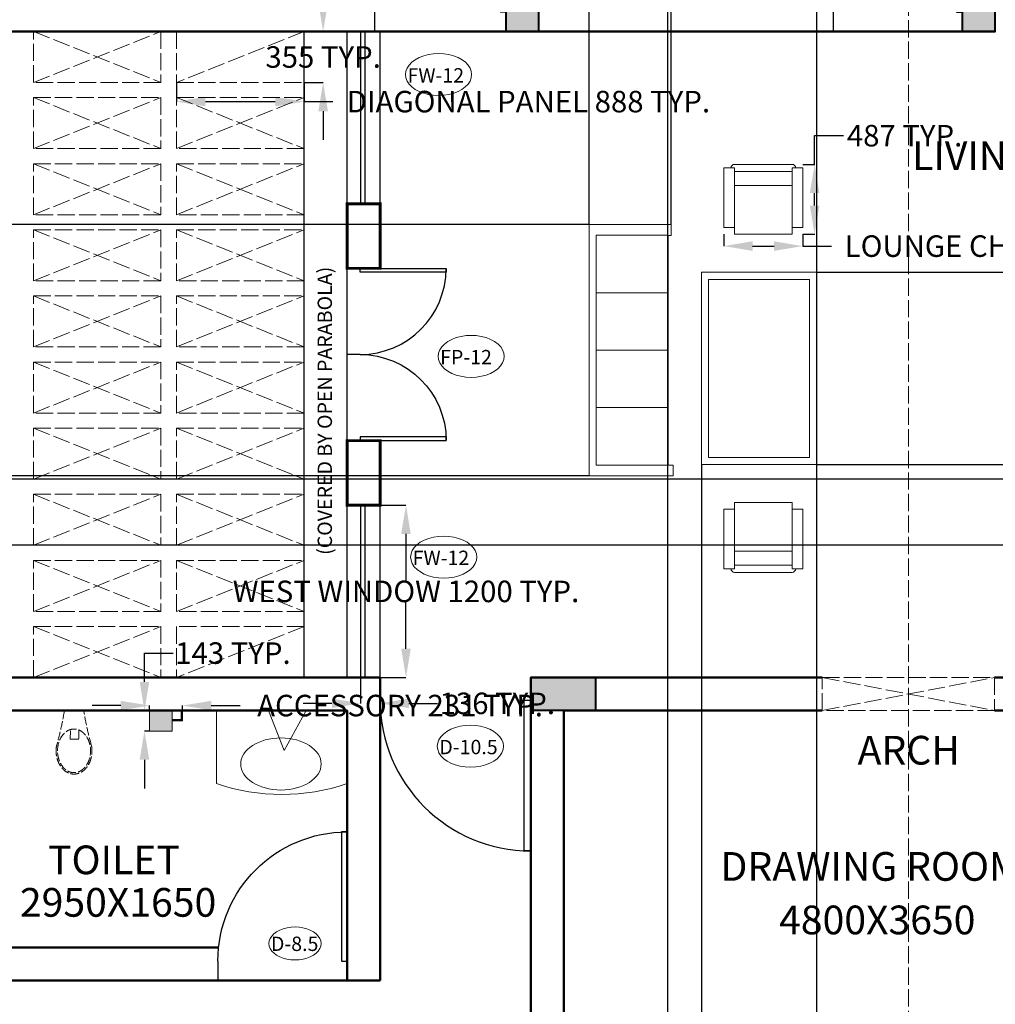
# Model space of a CAD drawing. Units: inches. Extents: x 22626 to 57351, y 2118 to 36234.
# Tile 4 of 10: x 34432 to 41227, y 16521 to 23379. Entities that reach past the tile are written whole.
import ezdxf

# ---------------------------------------------------------------- set-up
doc = ezdxf.new("R2010")
doc.units = ezdxf.units.IN
doc.header["$MEASUREMENT"] = 0
doc.linetypes.add('ACAD_ISO02W100', pattern=[15, 12, -3])
for name, color, linetype, lineweight in [('A-ANNO-DIMS', 130, 'Continuous', 18), ('A-ANNO-IDEN', 130, 'Continuous', 15), ('A-ANNO-TEXT', 130, 'Continuous', 18), ('A-AREA-IDEN', 130, 'Continuous', 18), ('A-COLS', 7, 'Continuous', 40), ('A-DOOR-OVHD', 32, 'ACAD_ISO02W100', 18), ('A-FLOR-FIXT', 30, 'Continuous', 18), ('A-FLOR-FIXT-HIDN', 30, 'ACAD_ISO02W100', 18), ('A-ROOF', 80, 'Continuous', 25), ('A-ROOF-OVHD', 80, 'ACAD_ISO02W100', 18), ('A-WALL', 80, 'Continuous', 50), ('DOORS', 32, 'Continuous', 25), ('FURNITURE', 30, 'Continuous', 18), ('WINDOWS', 212, 'Continuous', 25)]:
    doc.layers.add(name, color=color, linetype=linetype, lineweight=lineweight)
doc.layers.add('A-SECT', color=2, linetype='ACAD_ISO02W100', lineweight=18, true_color=0xf1eb1f)
doc.styles.get("Standard").update_dxf_attribs({"font": 'arial.ttf'})
doc.dimstyles.get("Standard").update_dxf_attribs({"dimtxt": 150, "dimasz": 200, "dimexe": 0.18, "dimexo": 0.0625, "dimgap": 0.09, "dimtad": 0, "dimtih": 1, "dimtoh": 1, "dimdec": 0, "dimzin": 0, "dimdsep": 46, "dimtxsty": 'Standard', "dimcen": 0.09, "dimadec": 0, "dimazin": 0, "dimtfac": 1, "dimtdec": 0, "dimtofl": 0, "dimtmove": 0, "dimatfit": 3, "dimfxl": 1, "dimtolj": 1, "dimtzin": 0, "dimarcsym": 0})

# ---------------------------------------------------------------- blocks, each defined once
blk = doc.blocks.new('*U7')
for p, q in [((0, 0), (-1e-16, -5.999999999999999)), ((40, -6e-16), (40, -6))]:
    blk.add_line(p, q)
blk.add_lwpolyline([(0, 0), (5.6e-15, 40), (1.750000000000007, 40), (1.749999999999998, -7e-16)], close=True)
blk.add_arc((0, 0), 40, 0, 90)
blk = doc.blocks.new('CHAIR-LOUNGE')
for p, q in [((475.0003983844144, 486.7758832616018), (75.00039838441444, 486.7758832616018)), ((0.0003983844144386, 47.37697057033074), (0.0003983844144386, 461.7758832616018)), ((75.00039838441444, 461.7758832616018), (0.0003983844144386, 461.7758832616018)), ((75.00039838441444, 461.7758832616018), (75.00039838441444, -4.78506444779e-05)), ((475.0003983844144, 436.7758832616018), (75.00039838441444, 436.7758832616018)), ((475.0003983844362, 461.7501739628424), (550.0003983844362, 461.7501739628424)), ((475.0003983844144, -4.78506444779e-05), (475.0003983844144, 461.750173962846)), ((550.0003983844144, 47.37697057033074), (550.0003983844144, 461.7501739628424)), ((75.00039838441444, 339.7687890747984), (475.0003983844144, 339.7687890747984)), ((75.00039838441444, 47.37697057033074), (0.0003983844144386, 47.37697057033074)), ((475.0003983844144, 47.37697057033074), (550.0003983844144, 47.37697057033074)), ((75.00039838440716, -4.78506481159e-05), (475.0003983844144, -4.78506481159e-05))]:
    blk.add_line(p, q)
for centre, start, end in [((75.00039838441444, 461.7758832616018), 90, 180), ((475.0003983844144, 461.7758832616018), 359.9410786171467, 90)]:
    blk.add_arc(centre, 25, start, end)
blk = doc.blocks.new('WC')
at = {"ltscale": 5}
for p, q in [((307.4540408789253, 157.9229967620813), (242.2174300020561, 157.9229967620813)), ((242.2174300020561, 157.9229967620813), (242.2174300020561, 97.87988847275483)), ((307.4540408789253, 157.9229967620813), (307.4540408789253, 157.9229967620813)), ((242.2174300020561, 97.87988847275483), (310.0842174796853, 99.70460823710528))]:
    blk.add_line(p, q, dxfattribs=at)
for centre, start, end in [((780.732508801062, 2286.288249576111), 254.000576969056, 260.8285458946419), ((780.732508801062, -2036.267674000785), 99.17145410535805, 105.999423030944)]:
    blk.add_arc(centre, 2121.236142909723, start, end, dxfattribs=at)
blk.add_ellipse((161.9027973060947, 125.0102877876634), major_axis=(151.9040759523413, 0), ratio=0.7571275708385353, start_param=-1.570796326794896, end_param=4.712388980384689, dxfattribs=at)
for points, knots in [([(196.0611207178517, 247.2193096078299), (189.9898489161132, 248.2266596507652), (183.8456655129121, 248.9650412442752), (168.6182293347155, 250.1102459839712), (159.4964975931143, 250.2034131541222), (141.3581357193834, 249.212698022955), (132.3417047420516, 248.1288311957833), (114.6613914742556, 244.8098406800164), (105.9976853845146, 242.5747636017513), (89.26201623554518, 237.0062334978611), (81.19018288652298, 233.6728365616509), (65.86452451616788, 225.9859897466813), (58.61077128878969, 221.6325587335632), (45.13156838521536, 212.0080719868456), (38.90616664764093, 206.7369257869286), (27.67640637096338, 195.4043234284545), (22.67220516936504, 189.3426231032536), (14.05759261523781, 176.5860631599644), (10.44766267286468, 169.8909471035294), (4.765577569938614, 156.0629077761186), (2.69424158098991, 148.9301527436837), (0.1846293913040426, 134.463597005164), (-0.2530317139462568, 127.1307025187488), (0.5271766823570943, 112.5265070110981), (1.744832412616233, 105.2563518462193), (5.77749157987273, 91.03263116568269), (8.591685077881264, 84.07962673572185), (15.69573821845551, 70.70922901844096), (19.98490811580268, 64.29173781119243), (29.87879523489392, 52.16900764399179), (35.483208879421, 46.46348057011346), (47.82439502190391, 35.90657261581146), (54.56108629030495, 31.05501885116246), (68.96556532807881, 22.32099587028279), (76.63330319123634, 18.43849746629348), (92.68186228567357, 11.73355477496807), (101.0625846676266, 8.91115468616772), (118.3043576900527, 4.392898517646244), (127.1652540279829, 2.697098106120392), (144.6597339432555, 0.5298149587142689), (153.2812269904534, -0.000476238605188), (161.9027973060947, -0.000476238605188)], [1.35503494441986, 1.35503494441986, 1.35503494441986, 1.35503494441986, 1.471789532681877, 1.471789532681877, 1.642812487519809, 1.642812487519809, 1.813835442357741, 1.813835442357741, 1.984858397195673, 1.984858397195673, 2.155881352033606, 2.155881352033606, 2.326904306871538, 2.326904306871538, 2.49792726170947, 2.49792726170947, 2.668950216547402, 2.668950216547402, 2.839973171385334, 2.839973171385334, 3.010996126223266, 3.010996126223266, 3.182019081061198, 3.182019081061198, 3.35304203589913, 3.35304203589913, 3.524064990737062, 3.524064990737062, 3.695087945574994, 3.695087945574994, 3.866110900412926, 3.866110900412926, 4.037133855250859, 4.037133855250859, 4.208156810088791, 4.208156810088791, 4.379179764926723, 4.379179764926723, 4.550202719764655, 4.550202719764655, 4.712388980384689, 4.712388980384689, 4.712388980384689, 4.712388980384689]), ([(161.9027973060947, -0.000476238605188), (167.8851873344465, -0.000476238605188), (173.8675648995122, 0.254611844480678), (185.2699231324077, 1.230286525809788), (190.6953945214336, 1.911114408936555), (196.0639028232108, 2.802063691000512)], [-1.570796326794896, -1.570796326794896, -1.570796326794896, -1.570796326794896, -1.458257493061962, -1.458257493061962, -1.355016516099114, -1.355016516099114, -1.355016516099114, -1.355016516099114])]:
    blk.add_open_spline(points, degree=3, knots=knots, dxfattribs=at)
blk = doc.blocks.new('VANITY-BASIN')
for p, q in [((584.7220439586453, 910.0402479339828), (75.43762569876708, 910.0402479339828)), ((305.8230790732414, 471.9850997598696), (584.7220439586453, 624.7406586797733)), ((305.8230790732414, 471.9850997598696), (584.7220439586453, 362.8739423048537))]:
    blk.add_line(p, q)
blk.add_arc((1409.991080111897, 455.0201781493488), 1409.991555504085, 161.1730336158717, 198.8269663841282)
blk.add_ellipse((212.5566461408889, 449.1359101998277), major_axis=(0, -280.3059750137254), ratio=0.6469075979310198)
blk = doc.blocks.new('COL-RECTANGULAR')
h = blk.add_hatch(color=256)
h.dxf.hatch_style = 1
h.paths.add_polyline_path([(4.39586474386e-05, 0.0001083647293854), (450.0000439586474, 0.0001083647293854), (450.0000439586474, 230.0001083647294), (4.39586474386e-05, 230.0001083647294)])
blk.add_lwpolyline([(4.39586474386e-05, 0.0001083647293854), (4.39586474386e-05, 230.0001083647294), (450.0000439586474, 230.0001083647294), (450.0000439586474, 0.0001083647293854)], close=True)
blk = doc.blocks.new('CANOPY-CROSSED-PANEL')
at = {"ltscale": 10}
for p, q in [((4.39586510765e-05, -7.7958175098e-06), (887.5000439586511, 355.3241083647299)), ((4.39586510765e-05, 355.3241083647299), (887.5000439586511, -7.7958175098e-06))]:
    blk.add_line(p, q, dxfattribs=at)
blk.add_lwpolyline([(4.39586510765e-05, 355.3241083647299), (887.5000439586511, 355.3241083647299), (887.5000439586511, -7.7958175098e-06), (4.39586510765e-05, -7.7958175098e-06)], close=True, dxfattribs=at)
blk = doc.blocks.new('BATH-WALL-ACCESSORY')
h = blk.add_hatch(color=256)
h.dxf.hatch_style = 1
h.paths.add_polyline_path([(142.8430439586445, 231.1050653827879), (71.42162994010141, 231.1050653827879), (71.42162994010141, 158.5160872540764), (81.4216299401014, 158.5160872540764), (81.42162994010869, 221.1050653827879), (142.8430439586445, 221.1050653827879)])
h = blk.add_hatch(color=256)
h.dxf.hatch_style = 1
h.paths.add_polyline_path([(142.8430439586445, 158.5160872540764), (0.0002159215582651, 158.5160872540764), (0.0002159215582651, -1.22242890939e-05), (142.8430439586445, -1.22242854559e-05)])
for p, q in [((71.42162994010141, 158.5160872540764), (71.42162994010141, 231.1050653827879)), ((71.42162994010141, 231.1050653827879), (142.8430439586445, 231.1050653827879)), ((81.42162994010869, 221.1050653827879), (142.8430439586445, 221.1050653827879)), ((81.4216299401014, 158.5160872540764), (81.42162994010869, 221.1050653827879)), ((142.8430439586445, 158.5160872540764), (0.0002159215582651, 158.5160872540764)), ((0.0002159215582651, 158.5160872540764), (0.0002159215582651, -1.22242890939e-05)), ((142.8430439586445, 158.5160872540764), (142.8430439586445, 158.5160872540764)), ((0.0002159215582651, -1.22242890939e-05), (142.8430439586445, -1.22242854559e-05))]:
    blk.add_line(p, q)
blk = doc.blocks.new('WIN-FIXED-1200-WEST')
for p, q in [((0.0004449870903045, 1200.000108364729), (0.0004449870903045, 0.0001083647293854)), ((30.0004449870903, 1200.000108364729), (30.0004449870903, 0.0001083647293854))]:
    blk.add_line(p, q)
blk.add_lwpolyline([(136.2710439586444, 0.0001083647293854), (136.2710439586444, 1200.000108364729)])
blk = doc.blocks.new('CANOPY-DIAGONAL-PANEL')
at = {"ltscale": 10}
blk.add_line((887.5000439586511, 355.3241083647299), (4.39586510765e-05, -7.7958175098e-06), dxfattribs=at)
blk.add_lwpolyline([(887.5000439586511, 355.3241083647299), (4.39586510765e-05, 355.3241083647299), (4.39586510765e-05, -7.7958175098e-06), (887.5000439586511, -7.7958175098e-06)], close=True, dxfattribs=at)
blk = doc.blocks.new('*D52')
at = {"layer": 'A-ANNO-DIMS', "color": 0, "lineweight": -2, "transparency": 16777216}
for p, q in [((35524.92904395865, 22941.47349220418), (35524.92904395865, 22808.23099220418)), ((36412.42904395865, 22941.47349220418), (36412.42904395865, 22808.23099220418)), ((35724.92904395865, 22808.41099220418), (36212.42904395865, 22808.41099220418)), ((36412.42904395865, 22808.41099220418), (36612.42904395865, 22808.41099220418))]:
    blk.add_line(p, q, dxfattribs=at)
at = {"layer": 'A-ANNO-DIMS', "color": 0, "transparency": 16777216}
for points in [[(35724.92904395865, 22841.74432553752), (35724.92904395865, 22775.07765887085), (35524.92904395865, 22808.41099220418)], [(36212.42904395865, 22841.74432553752), (36212.42904395865, 22775.07765887085), (36412.42904395865, 22808.41099220418)]]:
    blk.add_solid(points, dxfattribs=at)
at = {"layer": 'Defpoints', "color": 0, "transparency": 16777216}
for p in [(35524.92904395865, 22941.53599220418), (36412.42904395865, 22941.53599220418), (36412.42904395865, 22808.41099220418)]:
    blk.add_point(p, dxfattribs=at)
at = {"layer": 'A-ANNO-DIMS', "color": 0, "transparency": 16777216, "insert": (37975.41126769671, 22808.41099220418), "char_height": 150, "attachment_point": 5}
blk.add_mtext('\\A1;DIAGONAL PANEL 888 TYP.', dxfattribs=at)
blk = doc.blocks.new('*D53')
at = {"layer": 'A-ANNO-DIMS', "color": 0, "lineweight": -2, "transparency": 16777216}
for p, q in [((36545.55404395868, 23496.86010836474), (36545.55404395868, 23696.86010836474)), ((36412.49154395866, 23296.86010836474), (36545.73404395868, 23296.86010836474)), ((36412.49154395866, 22941.53599220419), (36545.73404395868, 22941.53599220419)), ((36545.55404395868, 22741.53599220419), (36545.55404395868, 22541.53599220419))]:
    blk.add_line(p, q, dxfattribs=at)
at = {"layer": 'A-ANNO-DIMS', "color": 0, "transparency": 16777216}
for points in [[(36512.22071062534, 23496.86010836474), (36578.88737729201, 23496.86010836474), (36545.55404395868, 23296.86010836474)], [(36512.22071062534, 22741.53599220419), (36578.88737729201, 22741.53599220419), (36545.55404395868, 22941.53599220419)]]:
    blk.add_solid(points, dxfattribs=at)
at = {"layer": 'Defpoints', "color": 0, "transparency": 16777216}
for p in [(36412.42904395866, 23296.86010836474), (36545.55404395868, 23296.86010836474), (36412.42904395866, 22941.53599220419)]:
    blk.add_point(p, dxfattribs=at)
at = {"layer": 'A-ANNO-DIMS', "color": 0, "transparency": 16777216, "insert": (36545.55404395868, 23119.19805028445), "char_height": 150, "attachment_point": 5}
blk.add_mtext('\\A1;355 TYP.', dxfattribs=at)
blk = doc.blocks.new('*D68')
at = {"layer": 'A-ANNO-DIMS', "color": 0, "lineweight": -2, "transparency": 16777216}
for p, q in [((35135.53720708872, 18601.52587000579), (34935.53720708872, 18601.52587000579)), ((35335.53720708872, 18566.92260836472), (35335.53720708872, 18601.70587000579)), ((35566.6422846958, 18566.92260836472), (35566.6422846958, 18601.70587000579)), ((35766.6422846958, 18601.52587000579), (35966.6422846958, 18601.52587000579))]:
    blk.add_line(p, q, dxfattribs=at)
at = {"layer": 'A-ANNO-DIMS', "color": 0, "transparency": 16777216}
for points in [[(35135.53720708872, 18634.85920333912), (35135.53720708872, 18568.19253667246), (35335.53720708872, 18601.52587000579)], [(35766.6422846958, 18634.85920333912), (35766.6422846958, 18568.19253667246), (35566.6422846958, 18601.52587000579)]]:
    blk.add_solid(points, dxfattribs=at)
at = {"layer": 'Defpoints', "color": 0, "transparency": 16777216}
for p in [(35566.6422846958, 18601.52587000579), (35335.53720708872, 18566.86010836472), (35566.6422846958, 18566.86010836472)]:
    blk.add_point(p, dxfattribs=at)
at = {"layer": 'A-ANNO-DIMS', "color": 0, "transparency": 16777216, "insert": (37081.44920147616, 18601.52587000579), "char_height": 150, "attachment_point": 5}
blk.add_mtext('\\A1;ACCESSORY 231 TYP.', dxfattribs=at)
blk = doc.blocks.new('*D69')
at = {"layer": 'A-ANNO-DIMS', "color": 0, "lineweight": -2, "transparency": 16777216}
for p, q in [((35300.87144544769, 18766.86010836473), (35300.87144544769, 18966.86010836473)), ((35300.87144544769, 18966.86010836473), (35500.87144544769, 18966.86010836473)), ((35335.47470708873, 18566.86010836473), (35300.69144544769, 18566.86010836473)), ((35335.47470708873, 18424.01728032765), (35300.69144544769, 18424.01728032765)), ((35300.87144544769, 18224.01728032765), (35300.87144544769, 18024.01728032765))]:
    blk.add_line(p, q, dxfattribs=at)
at = {"layer": 'A-ANNO-DIMS', "color": 0, "transparency": 16777216}
for points in [[(35267.53811211435, 18766.86010836473), (35334.20477878102, 18766.86010836473), (35300.87144544769, 18566.86010836473)], [(35267.53811211435, 18224.01728032765), (35334.20477878102, 18224.01728032765), (35300.87144544769, 18424.01728032765)]]:
    blk.add_solid(points, dxfattribs=at)
at = {"layer": 'Defpoints', "color": 0, "transparency": 16777216}
for p in [(35300.87144544769, 18566.86010836473), (35335.53720708873, 18566.86010836473), (35335.53720708873, 18424.01728032765)]:
    blk.add_point(p, dxfattribs=at)
at = {"layer": 'A-ANNO-DIMS', "color": 0, "transparency": 16777216, "insert": (35917.24725718029, 18966.86010836472), "char_height": 150, "attachment_point": 5}
blk.add_mtext('\\A1;143 TYP.', dxfattribs=at)
blk = doc.blocks.new('*D76')
at = {"layer": 'A-ANNO-DIMS', "color": 0, "lineweight": -2, "transparency": 16777216}
for p, q in [((39336.54639838442, 21884.32545214935), (39336.54639838442, 21801.70795214935)), ((39886.54639838444, 21884.32545214935), (39886.54639838444, 21801.70795214935)), ((39536.54639838442, 21801.88795214935), (39686.54639838444, 21801.88795214935)), ((39886.54639838444, 21801.88795214935), (40086.54639838444, 21801.88795214935))]:
    blk.add_line(p, q, dxfattribs=at)
at = {"layer": 'A-ANNO-DIMS', "color": 0, "transparency": 16777216}
for points in [[(39536.54639838442, 21835.22128548268), (39536.54639838442, 21768.55461881602), (39336.54639838442, 21801.88795214935)], [(39686.54639838444, 21835.22128548268), (39686.54639838444, 21768.55461881602), (39886.54639838444, 21801.88795214935)]]:
    blk.add_solid(points, dxfattribs=at)
at = {"layer": 'Defpoints', "color": 0, "transparency": 16777216}
for p in [(39336.54639838442, 21884.38795214935), (39886.54639838444, 21884.38795214935), (39886.54639838444, 21801.88795214935)]:
    blk.add_point(p, dxfattribs=at)
at = {"layer": 'A-ANNO-DIMS', "color": 0, "transparency": 16777216, "insert": (41333.34512962592, 21801.88795214935), "char_height": 150, "attachment_point": 5}
blk.add_mtext('\\A1;LOUNGE CHAIR 550 TYP.', dxfattribs=at)
blk = doc.blocks.new('*D77')
at = {"layer": 'A-ANNO-DIMS', "color": 0, "lineweight": -2, "transparency": 16777216}
for p, q in [((39969.04639838447, 22371.16388326161), (39969.04639838447, 22571.16388326161)), ((39969.04639838447, 22571.16388326161), (40169.04639838447, 22571.16388326161)), ((39886.60889838445, 22371.16388326161), (39969.22639838447, 22371.16388326161)), ((39969.04639838447, 22084.38795214936), (39969.04639838447, 22171.16388326161)), ((39886.60889838445, 21884.38795214936), (39969.22639838447, 21884.38795214936))]:
    blk.add_line(p, q, dxfattribs=at)
at = {"layer": 'A-ANNO-DIMS', "color": 0, "transparency": 16777216}
for points in [[(39935.71306505113, 22171.16388326161), (40002.3797317178, 22171.16388326161), (39969.04639838447, 22371.16388326161)], [(39935.71306505113, 22084.38795214936), (40002.3797317178, 22084.38795214936), (39969.04639838447, 21884.38795214936)]]:
    blk.add_solid(points, dxfattribs=at)
at = {"layer": 'Defpoints', "color": 0, "transparency": 16777216}
for p in [(39886.54639838446, 22371.16388326161), (39969.04639838447, 22371.16388326161), (39886.54639838446, 21884.38795214936)]:
    blk.add_point(p, dxfattribs=at)
at = {"layer": 'A-ANNO-DIMS', "color": 0, "transparency": 16777216, "insert": (40595.50065486468, 22571.1638832616), "char_height": 150, "attachment_point": 5}
blk.add_mtext('\\A1;487 TYP.', dxfattribs=at)
blk = doc.blocks.new('*D92')
at = {"layer": 'A-ANNO-DIMS', "color": 0, "lineweight": -2, "transparency": 16777216}
for p, q in [((36942.49154395866, 19996.86010836473), (37122.60904395868, 19996.86010836473)), ((37122.42904395868, 19796.86010836473), (37122.42904395868, 19474.55924888315)), ((37122.42904395868, 18996.86010836474), (37122.42904395868, 19319.16096784632)), ((36942.49154395866, 18796.86010836474), (37122.60904395868, 18796.86010836474))]:
    blk.add_line(p, q, dxfattribs=at)
at = {"layer": 'A-ANNO-DIMS', "color": 0, "transparency": 16777216}
for points in [[(37089.09571062534, 19796.86010836473), (37155.76237729201, 19796.86010836473), (37122.42904395868, 19996.86010836473)], [(37089.09571062534, 18996.86010836474), (37155.76237729201, 18996.86010836474), (37122.42904395868, 18796.86010836474)]]:
    blk.add_solid(points, dxfattribs=at)
at = {"layer": 'Defpoints', "color": 0, "transparency": 16777216}
for p in [(36942.42904395866, 19996.86010836473), (37122.42904395868, 19996.86010836473), (36942.42904395866, 18796.86010836474)]:
    blk.add_point(p, dxfattribs=at)
at = {"layer": 'A-ANNO-DIMS', "color": 0, "transparency": 16777216, "insert": (37122.42904395868, 19396.86010836472), "char_height": 150, "attachment_point": 5}
blk.add_mtext('\\A1;WEST WINDOW 1200 TYP.', dxfattribs=at)
blk = doc.blocks.new('*D93')
at = {"layer": 'A-ANNO-DIMS', "color": 0, "lineweight": -2, "transparency": 16777216}
for p, q in [((36806.1584449871, 18796.79760836473), (36806.1584449871, 18616.68010836473)), ((36942.42904395865, 18796.79760836473), (36942.42904395865, 18616.68010836473)), ((36606.1584449871, 18616.86010836473), (36406.1584449871, 18616.86010836473)), ((37142.42904395865, 18616.86010836473), (37342.42904395865, 18616.86010836473))]:
    blk.add_line(p, q, dxfattribs=at)
at = {"layer": 'A-ANNO-DIMS', "color": 0, "transparency": 16777216}
for points in [[(36606.1584449871, 18650.19344169806), (36606.1584449871, 18583.52677503139), (36806.1584449871, 18616.86010836473)], [(37142.42904395865, 18650.19344169806), (37142.42904395865, 18583.52677503139), (36942.42904395865, 18616.86010836473)]]:
    blk.add_solid(points, dxfattribs=at)
at = {"layer": 'Defpoints', "color": 0, "transparency": 16777216}
for p in [(36806.1584449871, 18796.86010836473), (36942.42904395865, 18796.86010836473), (36942.42904395865, 18616.86010836473)]:
    blk.add_point(p, dxfattribs=at)
at = {"layer": 'A-ANNO-DIMS', "color": 0, "transparency": 16777216, "insert": (37758.80485569126, 18616.86010836473), "char_height": 150, "attachment_point": 5}
blk.add_mtext('\\A1;136 TYP.', dxfattribs=at)
blk = doc.blocks.new('*D99')
at = {"layer": 'A-ANNO-DIMS', "color": 0, "lineweight": -2, "transparency": 16777216}
for p, q in [((41184.594559, 30456.86010800002), (57038.79342100006, 30456.86010800002)), ((57038.61342100005, 30256.86010800002), (57038.61342100005, 18933.58721577627)), ((57038.61342100006, 7456.860108000005), (57038.61342100005, 18780.13300022374)), ((43702.49154400001, 7256.860108000004), (57038.79342100006, 7256.860108000005))]:
    blk.add_line(p, q, dxfattribs=at)
at = {"layer": 'A-ANNO-DIMS', "color": 0, "transparency": 16777216}
for points in [[(57005.28008766672, 30256.86010800002), (57071.94675433339, 30256.86010800002), (57038.61342100005, 30456.86010800002)], [(57005.28008766673, 7456.860108000005), (57071.9467543334, 7456.860108000005), (57038.61342100006, 7256.860108000005)]]:
    blk.add_solid(points, dxfattribs=at)
at = {"layer": 'Defpoints', "color": 0, "transparency": 16777216}
for p in [(41184.53205900001, 30456.86010800002), (57038.61342100005, 30456.86010800002), (43702.42904400001, 7256.860108000004)]:
    blk.add_point(p, dxfattribs=at)
at = {"layer": 'A-ANNO-DIMS', "color": 0, "transparency": 16777216, "insert": (57038.61342100005, 18856.86010799999), "char_height": 150, "attachment_point": 5}
blk.add_mtext('\\A1;23200', dxfattribs=at)
blk = doc.blocks.new('*D100')
at = {"layer": 'A-ANNO-DIMS', "color": 0, "lineweight": -2, "transparency": 16777216}
for p, q in [((32057.429044, 23296.797608), (32057.429044, 2216.185148)), ((49187.429044, 23296.797608), (49187.429044, 2216.185148)), ((32257.429044, 2216.365148), (40347.407256824, 2216.365148)), ((48987.42904399999, 2216.365148), (40897.45083117598, 2216.365148))]:
    blk.add_line(p, q, dxfattribs=at)
at = {"layer": 'A-ANNO-DIMS', "color": 0, "transparency": 16777216}
for points in [[(32257.429044, 2249.698481333334), (32257.429044, 2183.031814666666), (32057.429044, 2216.365148)], [(48987.42904399999, 2249.698481333334), (48987.42904399999, 2183.031814666666), (49187.429044, 2216.365148)]]:
    blk.add_solid(points, dxfattribs=at)
at = {"layer": 'Defpoints', "color": 0, "transparency": 16777216}
for p in [(32057.429044, 23296.860108), (49187.429044, 23296.860108), (49187.429044, 2216.365148)]:
    blk.add_point(p, dxfattribs=at)
at = {"layer": 'A-ANNO-DIMS', "color": 0, "transparency": 16777216, "insert": (40622.42904399999, 2216.365148), "char_height": 150, "attachment_point": 5}
blk.add_mtext('\\A1;17130', dxfattribs=at)
blk = doc.blocks.new('*D104')
at = {"layer": 'A-ANNO-DIMS', "color": 0, "lineweight": -2, "transparency": 16777216}
for p, q in [((39180.506596, 20280.329385), (39180.506596, 2216.185148)), ((39982.977522, 20280.329385), (39982.977522, 2216.185148)), ((38980.506596, 2216.365148), (38780.506596, 2216.365148)), ((40182.977522, 2216.365148), (40382.977522, 2216.365148))]:
    blk.add_line(p, q, dxfattribs=at)
at = {"layer": 'A-ANNO-DIMS', "color": 0, "transparency": 16777216}
for points in [[(38980.506596, 2249.698481333334), (38980.506596, 2183.031814666666), (39180.506596, 2216.365148)], [(40182.977522, 2249.698481333334), (40182.977522, 2183.031814666666), (39982.977522, 2216.365148)]]:
    blk.add_solid(points, dxfattribs=at)
at = {"layer": 'Defpoints', "color": 0, "transparency": 16777216}
for p in [(39180.506596, 20280.391885), (39982.977522, 20280.391885), (39982.977522, 2216.365148)]:
    blk.add_point(p, dxfattribs=at)
at = {"layer": 'A-ANNO-DIMS', "color": 0, "transparency": 16777216, "insert": (39581.742059, 2216.365148), "char_height": 150, "attachment_point": 5}
blk.add_mtext('\\A1;802.5', dxfattribs=at)
blk = doc.blocks.new('*D105')
at = {"layer": 'A-ANNO-DIMS', "color": 0, "lineweight": -2, "transparency": 16777216}
for p, q in [((39983.04002200002, 21620.08858600001), (57038.79342100006, 21620.08858600001)), ((57038.61342100005, 21420.08858600001), (57038.61342100005, 21026.96734327627)), ((57038.61342100005, 20480.39188500001), (57038.61342100005, 20873.51312772375)), ((39983.04002200002, 20280.39188500001), (57038.79342100006, 20280.39188500001))]:
    blk.add_line(p, q, dxfattribs=at)
at = {"layer": 'A-ANNO-DIMS', "color": 0, "transparency": 16777216}
for points in [[(57005.28008766672, 21420.08858600001), (57071.94675433339, 21420.08858600001), (57038.61342100005, 21620.08858600001)], [(57005.28008766672, 20480.39188500001), (57071.94675433339, 20480.39188500001), (57038.61342100005, 20280.39188500001)]]:
    blk.add_solid(points, dxfattribs=at)
at = {"layer": 'Defpoints', "color": 0, "transparency": 16777216}
for p in [(39982.97752200002, 21620.08858600001), (57038.61342100005, 21620.08858600001), (39982.97752200002, 20280.39188500001)]:
    blk.add_point(p, dxfattribs=at)
at = {"layer": 'A-ANNO-DIMS', "color": 0, "transparency": 16777216, "insert": (57038.61342100005, 20950.24023549999), "char_height": 150, "attachment_point": 5}
blk.add_mtext('\\A1;1339.7', dxfattribs=at)
blk = doc.blocks.new('*D106')
at = {"layer": 'A-ANNO-DIMS', "color": 0, "lineweight": -2, "transparency": 16777216}
for p, q in [((38198.278783, 36136.059266), (37998.278783, 36136.059266)), ((38398.278783, 21952.121016), (38398.278783, 36136.239266)), ((38968.927296, 21952.121016), (38968.927296, 36136.239266)), ((39168.927296, 36136.059266), (39368.927296, 36136.059266))]:
    blk.add_line(p, q, dxfattribs=at)
at = {"layer": 'A-ANNO-DIMS', "color": 0, "transparency": 16777216}
for points in [[(38198.278783, 36169.39259933333), (38198.278783, 36102.72593266666), (38398.278783, 36136.059266)], [(39168.927296, 36169.39259933333), (39168.927296, 36102.72593266666), (38968.927296, 36136.059266)]]:
    blk.add_solid(points, dxfattribs=at)
at = {"layer": 'Defpoints', "color": 0, "transparency": 16777216}
for p in [(38968.927296, 36136.059266), (38398.278783, 21952.058516), (38968.927296, 21952.058516)]:
    blk.add_point(p, dxfattribs=at)
at = {"layer": 'A-ANNO-DIMS', "color": 0, "transparency": 16777216, "insert": (38683.6030395, 36136.059266), "char_height": 150, "attachment_point": 5}
blk.add_mtext('\\A1;570.6', dxfattribs=at)
blk = doc.blocks.new('*D107')
at = {"layer": 'A-ANNO-DIMS', "color": 0, "lineweight": -2, "transparency": 16777216}
for p, q in [((38398.21628300002, 21952.05851600001), (22909.89228600001, 21952.058516)), ((22910.07228600002, 21752.058516), (22910.07228600002, 21153.73446415826)), ((22910.07228600002, 20402.05851600001), (22910.07228600002, 21000.38256784175)), ((38398.21628300002, 20202.05851600001), (22909.89228600001, 20202.058516))]:
    blk.add_line(p, q, dxfattribs=at)
at = {"layer": 'A-ANNO-DIMS', "color": 0, "transparency": 16777216}
for points in [[(22876.73895266668, 21752.058516), (22943.40561933335, 21752.058516), (22910.07228600002, 21952.058516)], [(22876.73895266668, 20402.05851600001), (22943.40561933335, 20402.05851600001), (22910.07228600002, 20202.058516)]]:
    blk.add_solid(points, dxfattribs=at)
at = {"layer": 'Defpoints', "color": 0, "transparency": 16777216}
for p in [(22910.07228600002, 21952.058516), (38398.27878300002, 21952.05851600001), (38398.27878300002, 20202.05851600001)]:
    blk.add_point(p, dxfattribs=at)
at = {"layer": 'A-ANNO-DIMS', "color": 0, "transparency": 16777216, "insert": (22910.07228600002, 21077.058516), "char_height": 150, "attachment_point": 5}
blk.add_mtext('\\A1;1750', dxfattribs=at)
blk = doc.blocks.new('*D110')
at = {"layer": 'A-ANNO-DIMS', "color": 0, "lineweight": -2, "transparency": 16777216}
for p, q in [((38945.195609, 27402.749669), (38945.195609, 2216.185148)), ((39982.429044, 27402.749669), (39982.429044, 2216.185148)), ((39145.195609, 2216.365148), (39160.19231285744, 2216.365148)), ((39782.429044, 2216.365148), (39767.43234014257, 2216.365148))]:
    blk.add_line(p, q, dxfattribs=at)
at = {"layer": 'A-ANNO-DIMS', "color": 0, "transparency": 16777216}
for points in [[(39145.195609, 2249.698481333334), (39145.195609, 2183.031814666666), (38945.195609, 2216.365148)], [(39782.429044, 2249.698481333334), (39782.429044, 2183.031814666666), (39982.429044, 2216.365148)]]:
    blk.add_solid(points, dxfattribs=at)
at = {"layer": 'Defpoints', "color": 0, "transparency": 16777216}
for p in [(38945.195609, 27402.812169), (39982.429044, 27402.812169), (39982.429044, 2216.365148)]:
    blk.add_point(p, dxfattribs=at)
at = {"layer": 'A-ANNO-DIMS', "color": 0, "transparency": 16777216, "insert": (39463.8123265, 2216.365148), "char_height": 150, "attachment_point": 5}
blk.add_mtext('\\A1;1037.2', dxfattribs=at)
blk = doc.blocks.new('*D112')
at = {"layer": 'A-ANNO-DIMS', "color": 0, "lineweight": -2, "transparency": 16777216}
for p, q in [((22910.07228600002, 20178.418736), (22910.07228600002, 20378.418736)), ((22910.07228600002, 20378.418736), (23110.07228600002, 20378.418736)), ((45719.86654400001, 20178.41873600001), (22909.89228600001, 20178.418736)), ((22910.07228600002, 19917.899194), (22910.07228600002, 19978.418736)), ((45719.86654400001, 19717.89919400001), (22909.89228600001, 19717.899194))]:
    blk.add_line(p, q, dxfattribs=at)
at = {"layer": 'A-ANNO-DIMS', "color": 0, "transparency": 16777216}
for points in [[(22876.73895266668, 19978.418736), (22943.40561933335, 19978.418736), (22910.07228600002, 20178.418736)], [(22876.73895266668, 19917.899194), (22943.40561933335, 19917.899194), (22910.07228600002, 19717.899194)]]:
    blk.add_solid(points, dxfattribs=at)
at = {"layer": 'Defpoints', "color": 0, "transparency": 16777216}
for p in [(22910.07228600002, 20178.418736), (45719.929044, 20178.41873600001), (45719.929044, 19717.89919400001)]:
    blk.add_point(p, dxfattribs=at)
at = {"layer": 'A-ANNO-DIMS', "color": 0, "transparency": 16777216, "insert": (23366.83008954708, 20378.41873599999), "char_height": 150, "attachment_point": 5}
blk.add_mtext('\\A1;460.5', dxfattribs=at)

msp = doc.modelspace()

# ---------------------------------------------------------------- linework, layer by layer
at = {"layer": 'A-ANNO-IDEN'}
for centre, major_axis in [((37349.68857688256, 22996.57356606163), (230.2388321358037, 0)), ((37576.76965244917, 21033.80099818483), (230.2388321358037, 0)), ((37385.27909127975, 19635.76913223417), (230.2388321358037, 0)), ((37571.09958781945, 18317.89574295287), (230.2388321358037, 0)), ((36349.601266638, 16944.38465518176), (181.3320649818415, 0))]:
    msp.add_ellipse(centre, major_axis=major_axis, ratio=0.6342549732601661, start_param=-1.570796326794896, end_param=4.712388980384689, dxfattribs=at)
at = {"layer": 'A-DOOR-OVHD', "ltscale": 10}
for p, q in [((40022.42904395864, 18796.86010836473), (41222.42904395864, 18566.86010836473)), ((40022.42904395864, 18566.86010836473), (41222.42904395865, 18796.86010836473))]:
    msp.add_line(p, q, dxfattribs=at)
msp.add_lwpolyline([(40022.42904395864, 18796.86010836473), (41222.42904395865, 18796.86010836473), (41222.42904395864, 18566.86010836473), (40022.42904395864, 18566.86010836473), (40022.42904395864, 18796.86010836473)], dxfattribs=at)
at = {"layer": 'A-FLOR-FIXT'}
msp.add_line((35802.38890438939, 18566.86010836473), (35802.38890438939, 18057.57569010485), dxfattribs=at)
at = {"layer": 'A-ROOF'}
msp.add_lwpolyline([(36412.42904395865, 18796.86010836473), (36412.42904395865, 23296.86010836473)], dxfattribs=at)
at = {"layer": 'A-SECT', "ltscale": 10}
msp.add_line((40622.42904395865, 34176.07617998196), (40622.42904395865, 4176.34823413092), dxfattribs=at)
at = {"layer": 'A-WALL'}
for p, q in [((38047.42904395865, 23296.86010836473), (34317.42904395865, 23296.86010836473)), ((41227.42904395864, 23296.86010836473), (38047.42904395865, 23296.86010836473)), ((36942.42904395865, 18796.86010836473), (33562.42904395865, 18796.86010836473)), ((36942.42904395865, 16686.86010836473), (36942.42904395865, 18796.86010836473)), ((38222.42904395865, 14916.86010836473), (38222.42904395865, 18566.86010836473)), ((36942.42904395865, 16686.86010836473), (33792.42904395865, 16686.86010836473)), ((37992.42904395865, 13186.86010836473), (37992.42904395865, 16686.86010836473))]:
    msp.add_line(p, q, dxfattribs=at)
at = {"layer": 'A-WALL', "const_width": 20}
for points in [[(36712.42904395865, 22096.86010836473), (36942.42904395865, 22096.86010836473), (36942.42904395865, 21646.86010836473), (36712.42904395865, 21646.86010836473)], [(36712.42904395865, 19996.86010836473), (36942.42904395865, 19996.86010836473), (36942.42904395865, 20446.86010836473), (36712.42904395865, 20446.86010836473)]]:
    msp.add_lwpolyline(points, close=True, dxfattribs=at)
at = {"layer": 'A-WALL'}
for points in [[(40022.42904395864, 18796.86010836473), (37992.42904395865, 18796.86010836473)], [(37992.42904395865, 14686.86010836473), (37992.42904395865, 18796.86010836473)], [(43252.42904395865, 18796.86010836473), (41222.42904395864, 18796.86010836473)], [(36712.42904395865, 16686.86010836473), (36712.42904395865, 18566.86010836473), (33792.42904395865, 18566.86010836473), (33792.42904395865, 16916.86010836473)], [(40022.42904395864, 18566.86010836473), (38222.42904395865, 18566.86010836473)], [(43022.42904395864, 18566.86010836473), (41222.42904395864, 18566.86010836473)], [(35817.45697735544, 16916.86010836473), (33792.42904395865, 16916.86010836473)]]:
    msp.add_lwpolyline(points, dxfattribs=at)
at = {"layer": 'FURNITURE'}
for p, q in [((38948.27878268968, 21952.05851619681), (38398.27878268968, 21952.05851619681)), ((38398.27878268968, 21952.05851619681), (38398.27878268968, 21477.05851619681)), ((38948.27878268968, 21952.05851619681), (38968.92729571679, 21952.05851619681)), ((38968.92729571679, 21952.05851619681), (38968.92729571679, 21876.27346814839)), ((38948.27878268968, 21877.05851619681), (38448.27878268968, 21877.05851619681)), ((38448.27878268968, 21877.05851619681), (38448.27878268968, 21477.05851619681)), ((38948.27878268968, 21877.05851619681), (38948.27878268968, 20277.05851619681)), ((38968.92729571679, 21876.27346814839), (38948.27878268968, 21876.27346814839)), ((38398.27878268968, 21477.05851619681), (38398.27878268968, 21077.05851619681)), ((38448.27878268968, 21477.05851619681), (38948.27878268968, 21477.05851619681)), ((38448.27878268968, 21477.05851619681), (38448.27878268968, 21077.05851619681)), ((38398.27878268968, 21077.05851619682), (38398.27878268968, 20677.05851619682)), ((38448.27878268968, 21077.05851619681), (38948.27878268968, 21077.05851619682)), ((38448.27878268968, 21077.05851619682), (38448.27878268968, 20677.05851619682)), ((38398.27878268968, 20677.05851619682), (38398.27878268968, 20202.05851619682)), ((38448.27878268968, 20677.05851619682), (38948.27878268968, 20677.05851619682)), ((38448.27878268968, 20677.05851619682), (38448.27878268968, 20277.05851619681)), ((38448.27878268968, 20277.05851619681), (38948.27878268968, 20277.05851619681)), ((38948.27878268968, 20277.05851619681), (38983.65746258913, 20277.05851619681)), ((38983.65746258913, 20277.05851619681), (38983.65746258913, 20201.56469181593)), ((38398.27878268968, 20202.05851619682), (38948.27878268968, 20202.05851619682)), ((38983.65746258913, 20201.56469181593), (38948.27878268968, 20202.05851619682))]:
    msp.add_line(p, q, dxfattribs=at)
for points in [[(39180.50659591262, 21620.08858604966), (39982.97752201383, 21620.08858604966), (39982.97752201383, 20280.3918852049), (39180.50659591262, 20280.3918852049)], [(39230.50659591262, 21570.08858604966), (39932.97752201383, 21570.08858604966), (39932.97752201383, 20330.39188520489), (39230.50659591262, 20330.39188520489)]]:
    msp.add_lwpolyline(points, close=True, dxfattribs=at)
at = {"layer": 'WINDOWS'}
msp.add_lwpolyline([(36712.42904395865, 18796.86010836473), (36712.42904395865, 23296.86010836473)], dxfattribs=at)

# ---------------------------------------------------------------- block references
at = {"layer": 'A-COLS', "extrusion": (0, 0, -1), "zscale": -1, "rotation": 90}
for p in [(-37817.42893559392, 23296.86006440608), (-40997.4289355939, 23296.86006440608)]:
    msp.add_blockref('COL-RECTANGULAR', p, dxfattribs=at)
at = {"layer": 'A-COLS'}
msp.add_blockref('COL-RECTANGULAR', (37992.429, 18566.86), dxfattribs=at)
at = {"layer": 'A-FLOR-FIXT', "extrusion": (0, 0, -1), "zscale": -1, "rotation": 90}
for name, p in [('BATH-WALL-ACCESSORY', (-35335.53721931301, 18424.01706440608)), ('VANITY-BASIN', (-35802.38879602532, 17982.13806440608))]:
    msp.add_blockref(name, p, dxfattribs=at)
at = {"layer": 'A-FLOR-FIXT-HIDN', "extrusion": (0, 0, -1), "zscale": -1, "rotation": 90}
msp.add_blockref('WC', (-34685.34804938639, 18124.23006440375), dxfattribs=at)
at = {"layer": 'A-ROOF-OVHD'}
for name, p in [('CANOPY-CROSSED-PANEL', (34527.56352580819, 22941.536)), ('CANOPY-DIAGONAL-PANEL', (35524.929, 22941.536)), ('CANOPY-CROSSED-PANEL', (34527.56352580819, 22481.01645735117)), ('CANOPY-CROSSED-PANEL', (35524.92900000001, 22481.01645735117)), ('CANOPY-CROSSED-PANEL', (34527.56352580819, 22020.49691470234)), ('CANOPY-CROSSED-PANEL', (35524.92900000001, 22020.49691470234)), ('CANOPY-CROSSED-PANEL', (34527.56352580819, 21559.97737205352)), ('CANOPY-CROSSED-PANEL', (35524.92900000001, 21559.97737205352)), ('CANOPY-CROSSED-PANEL', (34527.56352580819, 21099.45782940469)), ('CANOPY-CROSSED-PANEL', (35524.92900000001, 21099.45782940469)), ('CANOPY-CROSSED-PANEL', (34527.56352580819, 20638.93828675586)), ('CANOPY-CROSSED-PANEL', (35524.92900000001, 20638.93828675586)), ('CANOPY-CROSSED-PANEL', (34527.56352580819, 20178.41874410703)), ('CANOPY-CROSSED-PANEL', (35524.92900000001, 20178.41874410703)), ('CANOPY-CROSSED-PANEL', (34527.56352580819, 19717.8992014582)), ('CANOPY-CROSSED-PANEL', (35524.92900000001, 19717.8992014582)), ('CANOPY-CROSSED-PANEL', (34527.56352580819, 19257.37965880937)), ('CANOPY-CROSSED-PANEL', (35524.92900000001, 19257.37965880937)), ('CANOPY-CROSSED-PANEL', (34527.56352580819, 18796.86011616055)), ('CANOPY-DIAGONAL-PANEL', (35524.929, 18796.86011616055))]:
    msp.add_blockref(name, p, dxfattribs=at)
at = {"layer": 'DOORS'}
for p, xscale, yscale, zscale in [((37817.42904395865, 23434.11010836473), -22.875, 22.875, 22.875), ((40997.42904395864, 23431.86010836473), -22.5, 22.5, 22.5), ((36712.42904395864, 16821.86010836473), -22.5, 22.5, 22.5)]:
    msp.add_blockref('*U7', p, dxfattribs=dict(at, xscale=xscale, yscale=yscale, zscale=zscale))
for p, xscale, yscale, zscale, rotation in [((36802.42904395865, 21646.86010836473), 15, 15, 15, 270), ((36802.42904395865, 20446.86010836473), -15, 15, 15, 270), ((37992.42904395865, 18639.36010836473), 26.25, 26.25, 26.25, 180)]:
    msp.add_blockref('*U7', p, dxfattribs=dict(at, xscale=xscale, yscale=yscale, zscale=zscale, rotation=rotation))
at = {"layer": 'FURNITURE'}
msp.add_blockref('CHAIR-LOUNGE', (39336.546, 21884.388), dxfattribs=at)
at = {"layer": 'FURNITURE', "extrusion": (0, 0, -1), "zscale": -1, "rotation": 180}
msp.add_blockref('CHAIR-LOUNGE', (-39336.546, 20016.09247125456), dxfattribs=at)
at = {"layer": 'WINDOWS'}
for p in [(36806.158, 22096.86), (36806.158, 18796.86)]:
    msp.add_blockref('WIN-FIXED-1200-WEST', p, dxfattribs=at)

# ---------------------------------------------------------------- texts
at = {"layer": 'A-ANNO-IDEN'}
for s, p in [('FW-12', (37133.39061900433, 22941.31361154905)), ('FP-12', (37360.47169457094, 20978.54104367224)), ('FW-12', (37168.98113340151, 19580.50917772158)), ('D-10.5', (37354.80162994122, 18262.63578844028)), ('D-8.5', (36181.98423330129, 16892.10228690643))]:
    msp.add_text(s, height=100, dxfattribs=at).set_placement(p)
at = {"layer": 'A-ANNO-TEXT'}
msp.add_text('(COVERED BY OPEN PARABOLA)', height=100, rotation=90, dxfattribs=at).set_placement((36606.96073067966, 19650.97858766166))
msp.add_text('ARCH', height=200, dxfattribs=at).set_placement((40268.31593293355, 18190.63683384524))
at = {"layer": 'A-AREA-IDEN'}
for s, p in [('LIVING DINING AREA', (40647.62954596056, 22330.97267428323)), ('TOILET', (34629.34227655845, 17426.84508650598)), ('DRAWING ROOM', (39313.18688753899, 17381.10026301192)), ('2950X1650', (34433.22928763816, 17130.75621793182)), ('4800X3650', (39721.34734618743, 17008.27361284928))]:
    msp.add_text(s, height=200, dxfattribs=at).set_placement(p)

# ---------------------------------------------------------------- dimensions: what is measured, and where the dimension line sits
at = {"layer": 'A-ANNO-DIMS'}
for base, p1, p2, override, picture, middle in [((38968.927296, 36136.059266), (38398.278783, 21952.058516), (38968.927296, 21952.058516), {"dimdec": 1, "dimlfac": 1, "dimrnd": 0, "dimzin": 0, "dimdsep": 46, "dimlunit": 2}, '*D106', (38683.6030395, 36136.059266)), ((39982.429044, 2216.365148), (38945.195609, 27402.812169), (39982.429044, 27402.812169), {"dimdec": 1, "dimlfac": 1, "dimrnd": 0, "dimzin": 0, "dimdsep": 46, "dimlunit": 2}, '*D110', (39463.8123265, 2216.365148)), ((49187.429044, 2216.365148), (32057.429044, 23296.860108), (49187.429044, 23296.860108), {"dimdec": 0, "dimlfac": 1, "dimrnd": 0, "dimzin": 0, "dimdsep": 46, "dimlunit": 2}, '*D100', (40622.42904399999, 2216.365148)), ((39982.977522, 2216.365148), (39180.506596, 20280.391885), (39982.977522, 20280.391885), {"dimdec": 1, "dimlfac": 1, "dimrnd": 0, "dimzin": 0, "dimdsep": 46, "dimlunit": 2}, '*D104', (39581.742059, 2216.365148))]:
    dim = msp.add_linear_dim(base=base, p1=p1, p2=p2, dimstyle='Standard', override=override, dxfattribs=at)
    dim.commit()
    dim.dimension.update_dxf_attribs({"geometry": picture, "text_midpoint": middle})
for base, p1, p2, override, picture, middle in [((57038.61342100005, 30456.86010800002), (43702.42904399999, 7256.860107999999), (41184.53205899999, 30456.860108), {"dimdec": 0, "dimlfac": 1, "dimrnd": 0, "dimzin": 0, "dimdsep": 46, "dimlunit": 2}, '*D99', (57038.61342100005, 18856.86010799999)), ((22910.07228600002, 21952.058516), (38398.278783, 20202.058516), (38398.278783, 21952.058516), {"dimdec": 0, "dimlfac": 1, "dimrnd": 0, "dimzin": 0, "dimdsep": 46, "dimlunit": 2}, '*D107', (22910.07228600002, 21077.058516)), ((57038.61342100005, 21620.08858600001), (39982.977522, 20280.391885), (39982.977522, 21620.088586), {"dimdec": 1, "dimlfac": 1, "dimrnd": 0, "dimzin": 0, "dimdsep": 46, "dimlunit": 2}, '*D105', (57038.61342100005, 20950.24023549999)), ((22910.07228600002, 20178.418736), (45719.929044, 19717.899194), (45719.929044, 20178.418736), {"dimdec": 1, "dimlfac": 1, "dimrnd": 0, "dimzin": 0, "dimdsep": 46, "dimlunit": 2}, '*D112', (23366.83008954708, 20378.41873599999))]:
    dim = msp.add_linear_dim(base=base, p1=p1, p2=p2, angle=90, dimstyle='Standard', override=override, dxfattribs=at)
    dim.commit()
    dim.dimension.update_dxf_attribs({"geometry": picture, "text_midpoint": middle})
for base, p1, p2, text, picture, middle in [((36545.55404395868, 23296.86010836474), (36412.42904395865, 22941.53599220418), (36412.42904395865, 23296.86010836473), '<> TYP.', '*D53', (36545.55404395868, 23119.19805028445)), ((39969.04639838447, 22371.16388326161), (39886.54639838444, 21884.38795214935), (39886.54639838444, 22371.1638832616), '<> TYP.', '*D77', (40595.50065486468, 22571.1638832616)), ((37122.42904395868, 19996.86010836473), (36942.42904395865, 18796.86010836473), (36942.42904395865, 19996.86010836473), 'WEST WINDOW <> TYP.', '*D92', (37122.42904395868, 19396.86010836472)), ((35300.87144544769, 18566.86010836473), (35335.53720708872, 18424.01728032764), (35335.53720708872, 18566.86010836472), '<> TYP.', '*D69', (35917.24725718029, 18966.86010836472))]:
    dim = msp.add_linear_dim(base=base, p1=p1, p2=p2, angle=90, text=text, dimstyle='Standard', override={"dimdec": 0, "dimlfac": 1, "dimrnd": 0, "dimzin": 0, "dimdsep": 46, "dimlunit": 2}, dxfattribs=at)
    dim.commit()
    dim.dimension.update_dxf_attribs({"geometry": picture, "text_midpoint": middle})
for base, p1, p2, text, picture, middle in [((36412.42904395865, 22808.41099220418), (35524.92904395865, 22941.53599220418), (36412.42904395865, 22941.53599220418), 'DIAGONAL PANEL <> TYP.', '*D52', (37975.41126769671, 22808.41099220418)), ((39886.54639838444, 21801.88795214935), (39336.54639838442, 21884.38795214935), (39886.54639838444, 21884.38795214935), 'LOUNGE CHAIR <> TYP.', '*D76', (41333.34512962592, 21801.88795214935)), ((35566.6422846958, 18601.52587000579), (35335.53720708872, 18566.86010836472), (35566.6422846958, 18566.86010836472), 'ACCESSORY <> TYP.', '*D68', (37081.44920147616, 18601.52587000579)), ((36942.42904395865, 18616.86010836473), (36806.1584449871, 18796.86010836473), (36942.42904395865, 18796.86010836473), '<> TYP.', '*D93', (37758.80485569126, 18616.86010836473))]:
    dim = msp.add_linear_dim(base=base, p1=p1, p2=p2, text=text, dimstyle='Standard', override={"dimdec": 0, "dimlfac": 1, "dimrnd": 0, "dimzin": 0, "dimdsep": 46, "dimlunit": 2}, dxfattribs=at)
    dim.commit()
    dim.dimension.update_dxf_attribs({"geometry": picture, "text_midpoint": middle})

doc.saveas('drawing.dxf')
